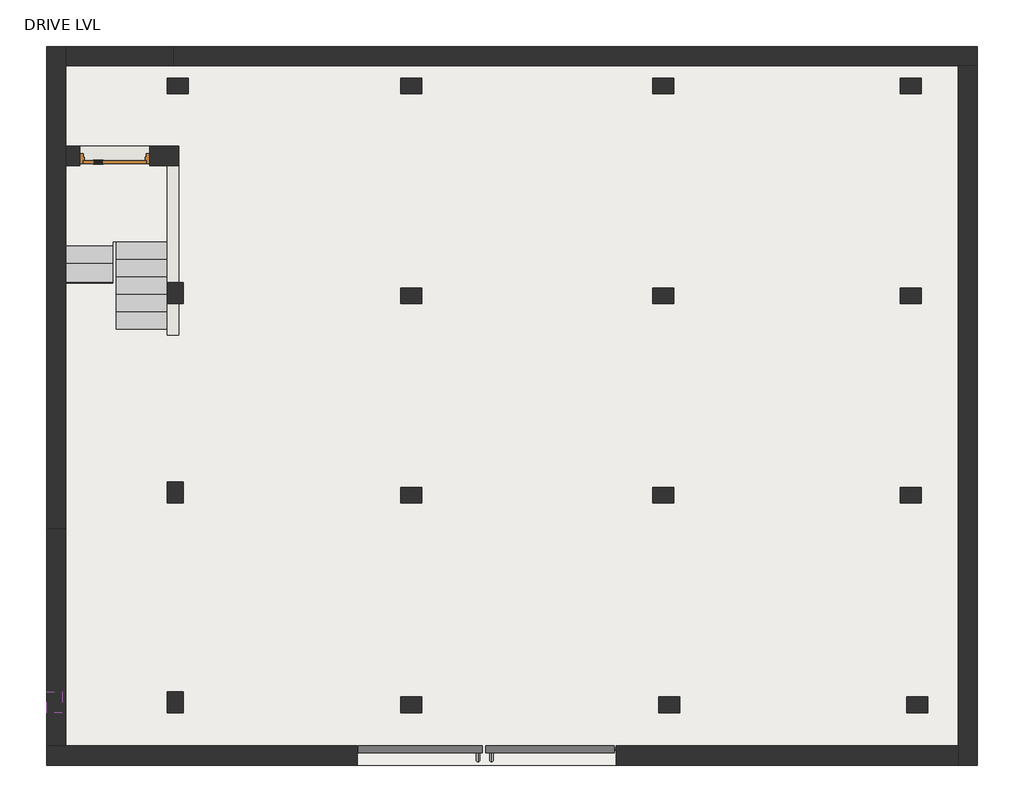
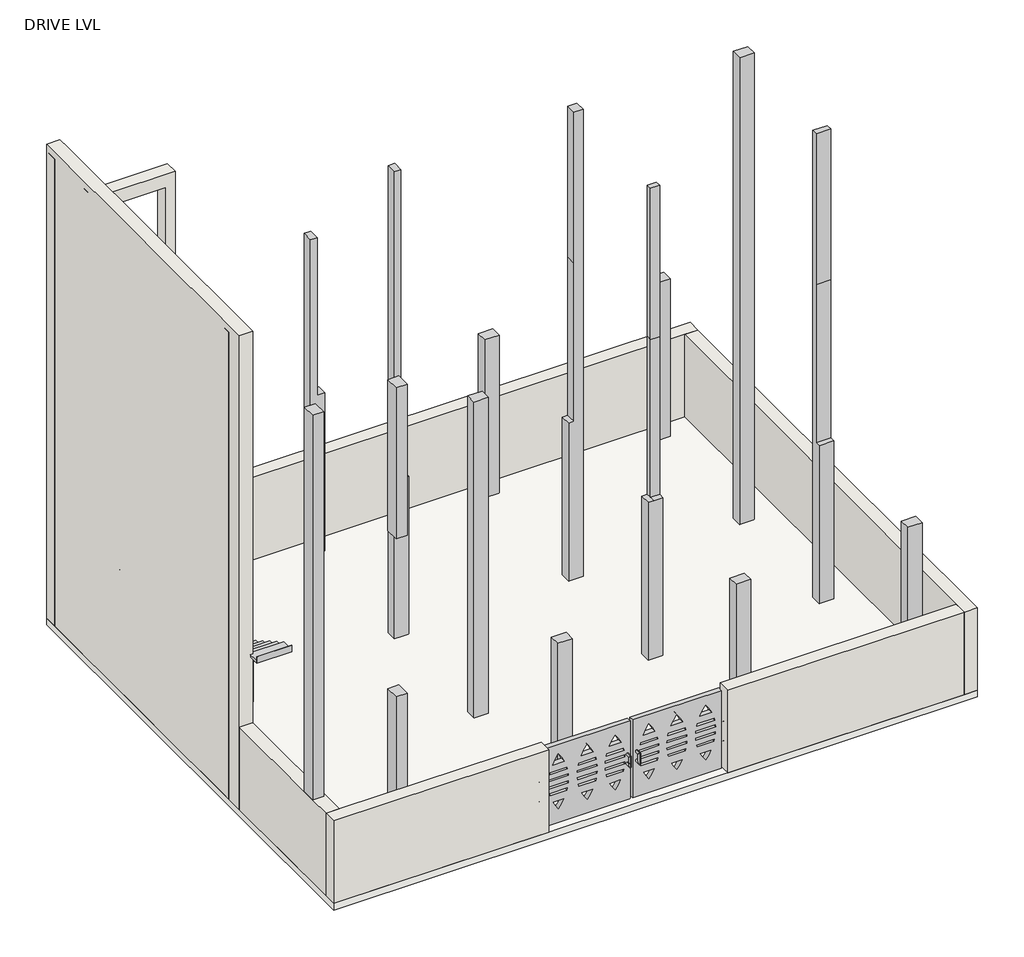
# One storey, incomplete: 21 columns, 8 walls, 2 slabs, 2 stair flights, 1 door, 1 proxy.
"""IFC4 building model written with IfcOpenShell, lengths in millimetres."""

from ifc_helpers import new_model, si_unit, frame, origin, origin_with_axes, place, context, project, spatial, polyline, outline, extrude, faceted_brep, transform, mapped, element, save
from components import generic_models_afecbd1f, column_4e4144c7, door_52fb15b9, non_monolithic_landing_83642a75, stair_flight_3ae1c9df, stair_flight_47155580

model = new_model("IFC4")

# Units and contexts
model_context = context("Model", 3, world=origin())
ifc_project = project(units=[si_unit("LENGTHUNIT", "METRE", prefix="MILLI")], contexts=[model_context])

# Site, building, storey
site = spatial("IfcSite", under=ifc_project)
building = spatial("IfcBuilding", under=site)
storey = spatial("IfcBuildingStorey", under=building, Name="DRIVE LVL", Elevation=0.0)

# Proxy
placement = place(None, origin())
generic_models_shape = generic_models_afecbd1f(model_context)
element("IfcBuildingElementProxy", 1, Name="Generic Models", at=placement, inside=storey, context=model_context, shape_type="MappedRepresentation", body=[
    mapped(generic_models_shape, transform((-1025.2155596, -1244.2923147, 0.0), x_axis=(1.0, 0.0, 0.0), y_axis=(0.0, 1.0, 0.0), z_axis=(0.0, 0.0, 1.0))),
])

# Columns
element("IfcColumn", 2, ObjectType="Rectangular Column : 24\" x 24\" 2", at=placement, inside=storey, context=model_context, shape_type="SweptSolid", body=[
    extrude(outline(polyline([(5711.1209761, -533.0923147), (5711.1209761, -761.6923147), (5406.3209761, -761.6923147), (5406.3209761, -533.0923147), (5711.1209761, -533.0923147)])), origin_with_axes(), (0.0, 0.0, 1.0), 3505.2),
])
element("IfcColumn", 3, ObjectType="Rectangular Column : 24\" x 24\" 2", at=placement, inside=storey, context=model_context, shape_type="SweptSolid", body=[
    extrude(outline(polyline([(2110.3088354, -533.0923147), (2110.3088354, -761.6923147), (1805.5088354, -761.6923147), (1805.5088354, -533.0923147), (2110.3088354, -533.0923147)])), origin_with_axes(), (0.0, 0.0, 1.0), 3505.2),
])
element("IfcColumn", 4, ObjectType="Rectangular Column : 24\" x 24\" 2", at=placement, inside=storey, context=model_context, shape_type="SweptSolid", body=[
    extrude(outline(polyline([(-1634.8155596, -533.0923147), (-1634.8155596, -761.6923147), (-1939.6155596, -761.6923147), (-1939.6155596, -533.0923147), (-1634.8155596, -533.0923147)])), origin_with_axes(), (0.0, 0.0, 1.0), 3505.2),
])
element("IfcColumn", 5, ObjectType="Rectangular Column : 24\" x 24\" 2", at=placement, inside=storey, context=model_context, shape_type="SweptSolid", body=[
    extrude(outline(polyline([(-1634.8155596, 2514.9076853), (-1634.8155596, 2286.3076853), (-1939.6155596, 2286.3076853), (-1939.6155596, 2514.9076853), (-1634.8155596, 2514.9076853)])), origin_with_axes(), (0.0, 0.0, 1.0), 7010.4),
])
element("IfcColumn", 6, ObjectType="Rectangular Column : 24\" x 24\" 2", at=placement, inside=storey, context=model_context, shape_type="SweptSolid", body=[
    extrude(outline(polyline([(0.0, -1939.6155596), (0.0, -1634.8155596), (3505.2, -1634.8155596), (3505.2, -1799.9155596), (7010.4, -1799.9155596), (10363.2, -1799.9155596), (10363.2, -1939.6155596), (0.0, -1939.6155596)])), frame((0.0, 5181.9076853, 0.0), z_axis=(0.0, 1.0, 0.0), x_axis=(0.0, 0.0, 1.0)), (0.0, 0.0, 1.0), 228.6),
])
element("IfcColumn", 7, ObjectType="Rectangular Column : 24\" x 24\" 2", at=placement, inside=storey, context=model_context, shape_type="SweptSolid", body=[
    extrude(outline(polyline([(0.0, 1717.9844404), (0.0, 2022.7844404), (10363.2, 2022.7844404), (10363.2, 1832.2844404), (7010.4, 1832.2844404), (3505.2, 1832.2844404), (3505.2, 1717.9844404), (0.0, 1717.9844404)])), frame((0.0, 5181.9076853, 0.0), z_axis=(0.0, 1.0, 0.0), x_axis=(0.0, 0.0, 1.0)), (0.0, 0.0, 1.0), 228.6),
])
element("IfcColumn", 8, ObjectType="Rectangular Column : 24\" x 24\" 2", at=placement, inside=storey, context=model_context, shape_type="SweptSolid", body=[
    extrude(outline(polyline([(2022.7844404, 8458.5076853), (2022.7844404, 8229.9076853), (1717.9844404, 8229.9076853), (1717.9844404, 8458.5076853), (2022.7844404, 8458.5076853)])), origin_with_axes(), (0.0, 0.0, 1.0), 3505.2),
])
element("IfcColumn", 9, ObjectType="Rectangular Column : 24\" x 24\" 2", at=placement, inside=storey, context=model_context, shape_type="SweptSolid", body=[
    extrude(outline(polyline([(0.0, -1939.6155596), (0.0, -1634.8155596), (3505.2, -1634.8155596), (3505.2, -1799.9155596), (7010.4, -1799.9155596), (7010.4, -1939.6155596), (0.0, -1939.6155596)])), frame((0.0, 8229.9076853, 0.0), z_axis=(0.0, 1.0, 0.0), x_axis=(0.0, 0.0, 1.0)), (0.0, 0.0, 1.0), 228.6),
])
element("IfcColumn", 10, ObjectType="Rectangular Column : 24\" x 24\" 2", at=placement, inside=storey, context=model_context, shape_type="SweptSolid", body=[
    extrude(outline(polyline([(0.0, -5330.5155596), (0.0, -5025.7155596), (7010.4, -5025.7155596), (7010.4, -5101.9155596), (3505.2, -5101.9155596), (3505.2, -5330.5155596), (0.0, -5330.5155596)])), frame((0.0, 8229.9076853, 0.0), z_axis=(0.0, 1.0, 0.0), x_axis=(0.0, 0.0, 1.0)), (0.0, 0.0, 1.0), 228.6),
])
element("IfcColumn", 11, ObjectType="Rectangular Column : 24\" x 24\" 2", at=placement, inside=storey, context=model_context, shape_type="SweptSolid", body=[
    extrude(outline(polyline([(-7083.1155596, 8915.7076853), (-6854.5155596, 8915.7076853), (-6854.5155596, 8610.9076853), (-7083.1155596, 8610.9076853), (-7083.1155596, 8915.7076853)])), origin_with_axes(), (0.0, 0.0, 1.0), 10363.2),
])
element("IfcColumn", 12, ObjectType="Rectangular Column : 24\" x 24\" 2", at=placement, inside=storey, context=model_context, shape_type="SweptSolid", body=[
    extrude(outline(polyline([(-7083.1155596, 7544.1076853), (-6854.5155596, 7544.1076853), (-6854.5155596, 7239.3076853), (-7083.1155596, 7239.3076853), (-7083.1155596, 7544.1076853)])), origin_with_axes(), (0.0, 0.0, 1.0), 10363.2),
])
element("IfcColumn", 13, ObjectType="Rectangular Column : 24\" x 24\" 2", at=placement, inside=storey, context=model_context, shape_type="SweptSolid", body=[
    extrude(outline(polyline([(0.0, -5101.9155596), (3505.2, -5101.9155596), (3505.2, -5330.5155596), (1066.8, -5330.5155596), (1066.8, -5165.4155596), (0.0, -5165.4155596), (0.0, -5101.9155596)])), frame((0.0, 5181.9076853, 0.0), z_axis=(0.0, 1.0, 0.0), x_axis=(0.0, 0.0, 1.0)), (0.0, 0.0, 1.0), 304.8),
])
element("IfcColumn", 14, ObjectType="Rectangular Column : 24\" x 24\" 2", at=placement, inside=storey, context=model_context, shape_type="SweptSolid", body=[
    extrude(outline(polyline([(-5330.5155596, 2591.1076853), (-5101.9155596, 2591.1076853), (-5101.9155596, 2286.3076853), (-5330.5155596, 2286.3076853), (-5330.5155596, 2591.1076853)])), origin_with_axes(), (0.0, 0.0, 1.0), 7010.4),
])
element("IfcColumn", 15, ObjectType="Rectangular Column : 24\" x 24\" 2", at=placement, inside=storey, context=model_context, shape_type="SweptSolid", body=[
    extrude(outline(polyline([(-7083.1155596, 2591.1076853), (-6854.5155596, 2591.1076853), (-6854.5155596, 2286.3076853), (-7083.1155596, 2286.3076853), (-7083.1155596, 2591.1076853)])), origin_with_axes(), (0.0, 0.0, 1.0), 10363.2),
])
element("IfcColumn", 16, ObjectType="Rectangular Column : 24\" x 24\" 2", at=placement, inside=storey, context=model_context, shape_type="Brep", body=[
    faceted_brep([(-7083.1155596, -456.8923147, 10363.2), (-6854.5155596, -456.8923147, 10363.2), (-6854.5155596, -456.8923147, 1828.8), (-7083.1155596, -456.8923147, 1828.8), (-7083.1155596, -456.8923147, 3505.2), (-7083.1155596, -456.8923147, 3810.0), (-7083.1155596, -456.8923147, 7010.4), (-7083.1155596, -456.8923147, 7315.2), (-6854.5155596, -761.6923147, 10363.2), (-6854.5155596, -761.6923147, 1828.8), (-7083.1155596, -761.6923147, 10363.2), (-7083.1155596, -761.6923147, 8077.2), (-7083.1155596, -761.6923147, 7010.4), (-7083.1155596, -761.6923147, 4572.0), (-7083.1155596, -761.6923147, 3505.2), (-7083.1155596, -761.6923147, 1828.8)], [[[0, 1, 2, 3, 4, 5, 6, 7]], [[1, 8, 9, 2]], [[8, 10, 11, 12, 13, 14, 15, 9]], [[10, 0, 7, 6, 5, 4, 3, 15, 14, 13, 12, 11]], [[1, 0, 10, 8]], [[3, 2, 9, 15]]]),
])
element("IfcColumn", 17, ObjectType="Rectangular Column : 24\" x 24\" 2", at=placement, inside=storey, context=model_context, shape_type="SweptSolid", body=[
    extrude(outline(polyline([(-5330.5155596, -456.8923147), (-5101.9155596, -456.8923147), (-5101.9155596, -761.6923147), (-5330.5155596, -761.6923147), (-5330.5155596, -456.8923147)])), origin_with_axes(), (0.0, 0.0, 1.0), 3505.2),
    extrude(outline(polyline([(-5330.5155596, -456.8923147), (-5101.9155596, -456.8923147), (-5101.9155596, -761.6923147), (-5330.5155596, -761.6923147), (-5330.5155596, -456.8923147)])), frame((0.0, 0.0, 7010.4), z_axis=(0.0, 0.0, 1.0), x_axis=(1.0, 0.0, 0.0)), (0.0, 0.0, 1.0), 3352.8),
])
element("IfcColumn", 18, ObjectType="Rectangular Column : 24\" x 24\" 2", at=placement, inside=storey, context=model_context, shape_type="SweptSolid", body=[
    extrude(outline(polyline([(2514.9076853, 0.0), (2286.3076853, 0.0), (2286.3076853, 3505.2), (2400.6076853, 3505.2), (2400.6076853, 7010.4), (2400.6076853, 10363.2), (2514.9076853, 10363.2), (2514.9076853, 0.0)])), frame((5307.0165832, 0.0, 0.0), z_axis=(1.0, 0.0, 0.0), x_axis=(0.0, 1.0, 0.0)), (0.0, 0.0, 1.0), 304.8),
])
element("IfcColumn", 19, ObjectType="Rectangular Column : 24\" x 24\" 2", at=placement, inside=storey, context=model_context, shape_type="SweptSolid", body=[
    extrude(outline(polyline([(5307.0165832, 8229.9076853), (5307.0165832, 8458.5076853), (5611.8165832, 8458.5076853), (5611.8165832, 8229.9076853), (5307.0165832, 8229.9076853)])), origin_with_axes(), (0.0, 0.0, 1.0), 3505.2),
])
element("IfcColumn", 20, ObjectType="Rectangular Column : 24\" x 24\" 2", at=placement, inside=storey, context=model_context, shape_type="Brep", body=[
    faceted_brep([(2022.7844404, 2514.9076853, 0.0), (2022.7844404, 2286.3076853, 0.0), (1717.9844404, 2286.3076853, 0.0), (1717.9844404, 2514.9076853, 0.0), (2022.7844404, 2514.9076853, 10363.2), (2022.7844404, 2400.6076853, 10363.2), (2022.7844404, 2400.6076853, 7010.4), (2022.7844404, 2400.6076853, 3505.2), (2022.7844404, 2286.3076853, 3505.2), (1717.9844404, 2514.9076853, 3505.2), (1832.2844404, 2514.9076853, 3505.2), (1832.2844404, 2514.9076853, 7010.4), (1832.2844404, 2514.9076853, 10363.2), (1832.2844404, 2400.6076853, 10363.2), (1832.2844404, 2400.6076853, 3505.2), (1832.2844404, 2400.6076853, 7010.4), (1717.9844404, 2286.3076853, 3505.2), (1832.2844404, 2286.3076853, 3505.2)], [[[0, 1, 2, 3]], [[1, 0, 4, 5, 6, 7, 8]], [[0, 3, 9, 10, 11, 12, 4]], [[4, 12, 13, 5]], [[11, 10, 14, 15]], [[16, 17, 14, 10, 9]], [[14, 7, 6, 15]], [[7, 14, 17, 8]], [[3, 2, 16, 9]], [[2, 1, 8, 17, 16]], [[12, 11, 15, 13]], [[6, 5, 13, 15]]]),
])
element("IfcColumn", 21, ObjectType="Rectangular Column : 24\" x 24\" 2", at=placement, inside=storey, context=model_context, shape_type="SweptSolid", body=[
    extrude(outline(polyline([(-1939.6155596, -761.6923147), (-1939.6155596, -533.0923147), (-1634.8155596, -533.0923147), (-1634.8155596, -761.6923147), (-1939.6155596, -761.6923147)])), origin_with_axes(), (0.0, 0.0, 1.0), 3505.2),
])
column_shape = column_4e4144c7(model_context)
element("IfcColumn", 22, ObjectType="Rectangular Column : 24\" x 24\" 2", at=placement, inside=storey, context=model_context, shape_type="MappedRepresentation", body=[
    mapped(column_shape, transform((5459.4165832, 5296.2076853, 0.0), x_axis=(-1.0, 0.0, 0.0), y_axis=(0.0, -1.0, 0.0), z_axis=(0.0, 0.0, 1.0))),
])

# Door
door_shape = door_52fb15b9(model_context)
element("IfcDoor", 23, ObjectType="Door-Passage-Single-Vision_Two_Lite : 36\" x 84\"", at=placement, inside=storey, context=model_context, shape_type="MappedRepresentation", body=[
    mapped(door_shape, transform((-6092.5155596, 7334.5576853, 825.5), x_axis=(1.0, 0.0, 0.0), y_axis=(0.0, 1.0, 0.0), z_axis=(0.0, 0.0, 1.0))),
])

# Slabs
element("IfcSlab", 24, ObjectType="Generic - 6\"", at=placement, inside=storey, context=model_context, shape_type="SweptSolid", body=[
    extrude(outline(polyline([(6429.6844404, 8915.7076853), (6429.6844404, -1523.6923147), (-7083.1155596, -1523.6923147), (-7083.1155596, 8915.7076853), (6429.6844404, 8915.7076853)])), frame((0.0, 0.0, -152.4), z_axis=(0.0, 0.0, 1.0), x_axis=(1.0, 0.0, 0.0)), (0.0, 0.0, 1.0), 152.4),
])
non_monolithic_landing_shape = non_monolithic_landing_83642a75(model_context)
element("IfcSlab", 25, ObjectType="Non-Monolithic Landing", at=placement, inside=storey, context=model_context, shape_type="MappedRepresentation", body=[
    mapped(non_monolithic_landing_shape, transform((0.0, 0.0, 0.0), x_axis=(1.0, 0.0, 0.0), y_axis=(0.0, 1.0, 0.0), z_axis=(0.0, 0.0, 1.0))),
])

# Stair flights
stair_flight_shape = stair_flight_3ae1c9df(model_context)
element("IfcStairFlight", 26, ObjectType="2\" Tread 1\" Nosing 1/4\" Riser", at=placement, inside=storey, context=model_context, shape_type="MappedRepresentation", body=[
    mapped(stair_flight_shape, transform((0.0, 0.0, 0.0), x_axis=(1.0, 0.0, 0.0), y_axis=(0.0, 1.0, 0.0), z_axis=(0.0, 0.0, 1.0))),
])
stair_flight_2_shape = stair_flight_47155580(model_context)
element("IfcStairFlight", 27, ObjectType="2\" Tread 1\" Nosing 1/4\" Riser", at=placement, inside=storey, context=model_context, shape_type="MappedRepresentation", body=[
    mapped(stair_flight_2_shape, transform((0.0, 0.0, 0.0), x_axis=(1.0, 0.0, 0.0), y_axis=(0.0, 1.0, 0.0), z_axis=(0.0, 0.0, 1.0))),
])

# Walls
element("IfcWall", 28, ObjectType="4", at=placement, inside=storey, context=model_context, shape_type="Brep", body=[
    faceted_brep([(-5330.5155596, 7188.5076853, 0.0), (-5330.5155596, 4727.0578046, 0.0), (-5330.5155596, 4727.0578046, 1066.8), (-5330.5155596, 5181.9076853, 1066.8), (-5330.5155596, 5486.7076853, 1066.8), (-5330.5155596, 7188.5076853, 1066.8), (-5165.4155596, 7188.5076853, 0.0), (-5165.4155596, 7188.5076853, 1066.8), (-5165.4155596, 5486.7076853, 1066.8), (-5165.4155596, 5181.9076853, 1066.8), (-5165.4155596, 4727.0578046, 1066.8), (-5165.4155596, 4727.0578046, 0.0), (-5165.4155596, 5181.9076853, 0.0), (-5165.4155596, 5486.7076853, 0.0)], [[[0, 1, 2, 3, 4, 5]], [[6, 7, 8, 9, 10, 11, 12, 13]], [[1, 0, 6, 13, 12, 11]], [[2, 1, 11, 10]], [[5, 4, 3, 2, 10, 9, 8, 7]], [[0, 5, 7, 6]]]),
])
element("IfcWall", 29, ObjectType="9", at=placement, inside=storey, context=model_context, shape_type="Brep", body=[
    faceted_brep([(-6803.7155596, 8636.3076853, 0.0), (-5241.6155596, 8636.3076853, 0.0), (-5241.6155596, 8636.3076853, 1828.8), (-5241.6155596, 8636.3076853, 3505.2), (-5101.9155596, 8636.3076853, 3505.2), (-5101.9155596, 8636.3076853, 7010.4), (-5381.3155596, 8636.3076853, 7010.4), (-6803.7155596, 8636.3076853, 7010.4), (-6803.7155596, 8915.7076853, 0.0), (-6803.7155596, 8915.7076853, 7010.4), (-5101.9155596, 8915.7076853, 7010.4), (-5101.9155596, 8915.7076853, 3505.2), (-5241.6155596, 8915.7076853, 3505.2), (-5241.6155596, 8915.7076853, 1828.8), (-5241.6155596, 8915.7076853, 0.0), (-5101.9155596, 8750.6076853, 7010.4), (-5101.9155596, 8750.6076853, 3505.2)], [[[0, 1, 2, 3, 4, 5, 6, 7]], [[8, 9, 10, 11, 12, 13, 14]], [[1, 0, 8, 14]], [[7, 6, 5, 15, 10, 9]], [[0, 7, 9, 8]], [[3, 2, 1, 14, 13, 12]], [[11, 16, 4, 3, 12]], [[5, 4, 16, 11, 10, 15]]]),
])
element("IfcWall", 30, ObjectType="9", at=placement, inside=storey, context=model_context, shape_type="Brep", body=[
    faceted_brep([(-6803.7155596, 7188.5076853, 0.0), (-5330.5155596, 7188.5076853, 0.0), (-5165.4155596, 7188.5076853, 0.0), (-5165.4155596, 7188.5076853, 1066.8), (-5165.4155596, 7188.5076853, 3505.2), (-5381.3155596, 7188.5076853, 3505.2), (-5381.3155596, 7188.5076853, 10364.7228861), (-6803.7155596, 7188.5076853, 10364.7228861), (-5584.5155596, 7188.5076853, 6565.9), (-5584.5155596, 7188.5076853, 4330.7), (-6600.5155596, 7188.5076853, 4330.7), (-6600.5155596, 7188.5076853, 6565.9), (-5584.5155596, 7188.5076853, 3060.7), (-5584.5155596, 7188.5076853, 825.5), (-6600.5155596, 7188.5076853, 825.5), (-6600.5155596, 7188.5076853, 3060.7), (-5584.5155596, 7188.5076853, 10071.1), (-5584.5155596, 7188.5076853, 7835.9), (-6600.5155596, 7188.5076853, 7835.9), (-6600.5155596, 7188.5076853, 10071.1), (-5165.4155596, 7467.9076853, 0.0), (-6803.7155596, 7467.9076853, 0.0), (-6803.7155596, 7467.9076853, 10364.7228861), (-5381.3155596, 7467.9076853, 10364.7228861), (-5381.3155596, 7467.9076853, 3505.2), (-5165.4155596, 7467.9076853, 3505.2), (-5584.5155596, 7467.9076853, 4330.7), (-5584.5155596, 7467.9076853, 6565.9), (-6600.5155596, 7467.9076853, 6565.9), (-6600.5155596, 7467.9076853, 4330.7), (-5584.5155596, 7467.9076853, 825.5), (-5584.5155596, 7467.9076853, 3060.7), (-6600.5155596, 7467.9076853, 3060.7), (-6600.5155596, 7467.9076853, 825.5), (-5584.5155596, 7467.9076853, 7835.9), (-5584.5155596, 7467.9076853, 10071.1), (-6600.5155596, 7467.9076853, 10071.1), (-6600.5155596, 7467.9076853, 7835.9)], [[[0, 1, 2, 3, 4, 5, 6, 7], [8, 9, 10, 11], [12, 13, 14, 15], [16, 17, 18, 19]], [[20, 21, 22, 23, 24, 25], [26, 27, 28, 29], [30, 31, 32, 33], [34, 35, 36, 37]], [[2, 1, 0, 21, 20]], [[7, 6, 23, 22]], [[0, 7, 22, 21]], [[26, 9, 8, 27]], [[27, 8, 11, 28]], [[28, 11, 10, 29]], [[9, 26, 29, 10]], [[31, 30, 13, 12]], [[32, 31, 12, 15]], [[33, 32, 15, 14]], [[30, 33, 14, 13]], [[35, 34, 17, 16]], [[36, 35, 16, 19]], [[37, 36, 19, 18]], [[34, 37, 18, 17]], [[5, 4, 25, 24]], [[2, 20, 25, 4, 3]], [[23, 6, 5, 24]]]),
])
element("IfcWall", 31, ObjectType="9", at=placement, inside=storey, context=model_context, shape_type="Brep", body=[
    faceted_brep([(-5241.6155596, 8636.3076853, 0.0), (6150.2844404, 8636.3076853, 0.0), (6429.6844404, 8636.3076853, 0.0), (6429.6844404, 8636.3076853, 1828.8), (6150.2844404, 8636.3076853, 1828.8), (-5241.6155596, 8636.3076853, 1828.8), (-5241.6155596, 8915.7076853, 0.0), (-5241.6155596, 8915.7076853, 1828.8), (6429.6844404, 8915.7076853, 1828.8), (6429.6844404, 8915.7076853, 0.0)], [[[0, 1, 2, 3, 4, 5]], [[6, 7, 8, 9]], [[2, 1, 0, 6, 9]], [[5, 4, 3, 8, 7]], [[0, 5, 7, 6]], [[3, 2, 9, 8]]]),
])
element("IfcWall", 32, ObjectType="9", at=placement, inside=storey, context=model_context, shape_type="Brep", body=[
    faceted_brep([(6150.2844404, 8636.3076853, 0.0), (6150.2844404, -1244.2923147, 0.0), (6150.2844404, -1523.6923147, 0.0), (6150.2844404, -1523.6923147, 1828.8), (6150.2844404, -1244.2923147, 1828.8), (6150.2844404, 8636.3076853, 1828.8), (6429.6844404, 8636.3076853, 0.0), (6429.6844404, 8636.3076853, 1828.8), (6429.6844404, -1523.6923147, 1828.8), (6429.6844404, -1523.6923147, 0.0)], [[[0, 1, 2, 3, 4, 5]], [[6, 7, 8, 9]], [[2, 1, 0, 6, 9]], [[5, 4, 3, 8, 7]], [[0, 5, 7, 6]], [[3, 2, 9, 8]]]),
])
element("IfcWall", 33, ObjectType="9", at=placement, inside=storey, context=model_context, shape_type="Brep", body=[
    faceted_brep([(6150.2844404, -1244.2923147, 1828.8), (6150.2844404, -1244.2923147, 0.0), (1189.6442362, -1244.2923147, 0.0), (1189.6442362, -1244.2923147, 1828.8), (6150.2844404, -1523.6923147, 0.0), (6150.2844404, -1523.6923147, 1828.8), (1189.6442362, -1523.6923147, 1828.8), (1189.6442362, -1523.6923147, 0.0)], [[[0, 1, 2, 3]], [[4, 5, 6, 7]], [[1, 4, 7, 2]], [[5, 0, 3, 6]], [[1, 0, 5, 4]], [[3, 2, 7, 6]]]),
    faceted_brep([(-7083.1155596, -1244.2923147, 0.0), (-7083.1155596, -1244.2923147, 1828.8), (-6803.7155596, -1244.2923147, 1828.8), (-2569.5557638, -1244.2923147, 1828.8), (-2569.5557638, -1244.2923147, 0.0), (-6803.7155596, -1244.2923147, 0.0), (-7083.1155596, -1523.6923147, 1828.8), (-7083.1155596, -1523.6923147, 0.0), (-2569.5557638, -1523.6923147, 0.0), (-2569.5557638, -1523.6923147, 1828.8)], [[[0, 1, 2, 3, 4, 5]], [[6, 7, 8, 9]], [[7, 0, 5, 4, 8]], [[1, 6, 9, 3, 2]], [[1, 0, 7, 6]], [[4, 3, 9, 8]]]),
])
element("IfcWall", 34, ObjectType="9", at=placement, inside=storey, context=model_context, shape_type="Brep", body=[
    faceted_brep([(-6803.7155596, -1244.2923147, 0.0), (-6803.7155596, 1905.3076853, 0.0), (-6803.7155596, 1905.3076853, 1828.8), (-6803.7155596, -1244.2923147, 1828.8), (-7083.1155596, -1244.2923147, 0.0), (-7083.1155596, -1244.2923147, 1828.8), (-7083.1155596, -761.6923147, 1828.8), (-7083.1155596, -456.8923147, 1828.8), (-7083.1155596, 1905.3076853, 1828.8), (-7083.1155596, 1905.3076853, 0.0)], [[[0, 1, 2, 3]], [[4, 5, 6, 7, 8, 9]], [[1, 0, 4, 9]], [[2, 1, 9, 8]], [[3, 2, 8, 7, 6, 5]], [[0, 3, 5, 4]]]),
])
element("IfcWall", 35, ObjectType="9 2", at=placement, inside=storey, context=model_context, shape_type="Brep", body=[
    faceted_brep([(-7083.1155596, 8915.7076853, 10515.6), (-7083.1155596, 8915.7076853, 0.0), (-7083.1155596, 1905.3076853, 0.0), (-7083.1155596, 1905.3076853, 1828.8), (-7083.1155596, 1905.3076853, 3505.2), (-7083.1155596, 1905.3076853, 3810.0), (-7083.1155596, 1905.3076853, 7010.4), (-7083.1155596, 1905.3076853, 7315.2), (-7083.1155596, 1905.3076853, 10515.6), (-6803.7155596, 8915.7076853, 0.0), (-6803.7155596, 8915.7076853, 7010.4), (-6803.7155596, 8915.7076853, 10515.6), (-6803.7155596, 8636.3076853, 10515.6), (-6803.7155596, 1905.3076853, 10515.6), (-6803.7155596, 1905.3076853, 1828.8), (-6803.7155596, 1905.3076853, 0.0), (-6803.7155596, 7188.5076853, 0.0), (-6803.7155596, 7467.9076853, 0.0), (-6803.7155596, 8636.3076853, 0.0)], [[[0, 1, 2, 3, 4, 5, 6, 7, 8]], [[9, 10, 11, 12, 13, 14, 15, 16, 17, 18]], [[2, 1, 9, 18, 17, 16, 15]], [[0, 8, 13, 12, 11]], [[0, 11, 10, 9, 1]], [[2, 15, 14, 13, 8, 7, 6, 5, 4, 3]]]),
])

save(model, "model.ifc")

# Revit data of these elements
# Type
#   Default Elevation = 0
# Type "Rectangular Column : 24\" x 24\" 2"
#   Assembly Code = "B1010200"
#   Depth = 0' - 9"
#   Offset Base = 0' - 0"
#   Offset Top = 0' - 0"
#   Width = 1' - 0"
#   Material = none
# Type "Door-Passage-Single-Vision_Two_Lite : 36\" x 84\""
#   Type Mark = "9"
#   Assembly Code = "B2030100"
#   Analytic Construction = "Wooden"
#   Thickness = 0' - 1 3/4"
#   Thermal Resistance (R) = 2.5876 (h·ft²·°F)/BTU
#   Swing Angle [instance default] = 90.00°
#   Strike Height = 3' - 4"
#   Rough Width [instance default] = 3' - 4"
#   Rough Height [instance default] = 7' - 4"
#   MF Opening Height [instance default] = 0' - 4"
#   MF Opening Width [instance default] = 0' - 4"
#   Heat Transfer Coefficient (U) = 0.3865 BTU/(h·ft²·°F)
#   Inset Calculate [instance default] = 0' - 4"
#   Masonry Inset [instance default] = 0' - 1"
#   Height = 7' - 0"
#   Width = 3' - 0"
#   Masonry Frame Depth = 0' - 5 3/4"
#   Masonry Frame [instance default] = yes
#   Function = 1
#   Dry Wall Frame [instance default] = no
#   Panel Material = Wood - Birch
#   Glazing = Glass
#   Glass Stop Material = Metal - Paint Finish - Grey
#   Frame Material = Metal - Paint Finish - Grey
#   Door Handle Material = Aluminum
#   Visual Light Transmittance = 0
#   Solar Heat Gain Coefficient = 0
#   Wall Closure = (empty or 0)
# Type "Generic - 6\""
#   Assembly Code = "B1010"
#   Function = 0
#   Layers, outside or top first: 0' - 6" no material (function 1)
# Type "4"
#   Assembly Code = "B2010"
#   Layers, outside or top first: 0' - 1" "Gypsum Wall Board" (function 1); 0' - 4 1/2" no material (function 1); 0' - 1" "Gypsum Wall Board" (function 1)
# Type "9"
#   Assembly Code = "B2010"
#   Layers, outside or top first: 0' - 1" "Gypsum Wall Board" (function 1); 0' - 9" no material (function 1); 0' - 1" "Gypsum Wall Board" (function 1)
# Type "9 2"
#   Assembly Code = "B2010"
#   Layers, outside or top first: 0' - 1" "Gypsum Wall Board" (function 1); 0' - 9" no material (function 1); 0' - 1" "Gypsum Wall Board" (function 1)
# Element 1 (IfcBuildingElementProxy)
#   Phase Created = New Construction
#   Materials on its faces: "GATE"
# Elements 2, 3, 4, 5, 6, 7, 8, 9, 10, 13, 14, 16, 17, 18, 19, 20, 21 (IfcColumn, "Rectangular Column : 24\" x 24\" 2")
#   Phase Created = New Construction
#   Materials on its faces: "Gypsum Wall Board", "Default Wall"
# Elements 11, 12, 15, 22 (IfcColumn, "Rectangular Column : 24\" x 24\" 2")
#   Phase Created = New Construction
# Element 23 (IfcDoor, "Door-Passage-Single-Vision_Two_Lite : 36\" x 84\"")
#   Swing Angle = 90.00°
#   Rough Width = 3' - 4"
#   Rough Height = 7' - 4"
#   Masonry Inset = 0' - 1"
#   MF Opening Width = 0' - 4"
#   MF Opening Height = 0' - 4"
#   Inset Calculate = 0' - 4"
#   Masonry Frame = yes
#   Dry Wall Frame = no
#   Phase Created = New Construction
#   Materials on its faces: "Metal - Paint Finish - Grey", "Aluminum", "Wood - Birch", "Glass"
# Element 24 (IfcSlab, "Generic - 6\"")
#   Height Offset From Level = 0' - 0"
#   Phase Created = New Construction
#   Materials on its faces: "Default Floor"
# Element 25 (IfcSlab, "Non-Monolithic Landing")
#   Phase Created = New Construction
# Elements 26, 27 (IfcStairFlight, "2\" Tread 1\" Nosing 1/4\" Riser")
#   Phase Created = New Construction
# Element 28 (IfcWall, "4")
#   Top Offset = 0' - 0"
#   Base Offset = 0' - 0"
#   Unconnected Height = 3' - 6"
#   wall height = 3' - 6"
#   Phase Created = New Construction
#   Base Constraint = DRIVE LVL
#   Materials on its faces: "Default Wall", "Gypsum Wall Board"
# Element 29 (IfcWall, "9")
#   Top Offset = 0' - 0"
#   Base Offset = 0' - 0"
#   wall height = 23' - 0"
#   Phase Created = New Construction
#   Base Constraint = DRIVE LVL
#   Top Constraint = SECOND FLOOR LVL
#   Materials on its faces: "Default Wall", "Gypsum Wall Board"
# Element 30 (IfcWall, "9")
#   Top Offset = -0' - 5.94004"
#   Base Offset = 0' - 0"
#   wall height = 34' - 0.05996"
#   Phase Created = New Construction
#   Base Constraint = DRIVE LVL
#   Top Constraint = ROOF LVL
#   Materials on its faces: "Default Wall", "Gypsum Wall Board"
# Elements 31, 32 (IfcWall, "9")
#   Top Offset = 0' - 0"
#   Base Offset = 0' - 0"
#   Unconnected Height = 6' - 0"
#   wall height = 6' - 0"
#   Phase Created = New Construction
#   Base Constraint = DRIVE LVL
#   Materials on its faces: "Gypsum Wall Board", "Default Wall"
# Elements 33, 34 (IfcWall, "9")
#   Top Offset = 0' - 0"
#   Base Offset = 0' - 0"
#   Unconnected Height = 6' - 0"
#   wall height = 6' - 0"
#   Phase Created = New Construction
#   Base Constraint = DRIVE LVL
#   Materials on its faces: "Default Wall", "Gypsum Wall Board"
# Element 35 (IfcWall, "9 2")
#   Top Offset = 0' - 0"
#   Base Offset = 0' - 0"
#   wall height = 34' - 6"
#   Phase Created = New Construction
#   Base Constraint = DRIVE LVL
#   Top Constraint = ROOF LVL
#   Materials on its faces: "Gypsum Wall Board", "Default Wall"
# Materials
#   "Wood - Birch": class "Wood", colour RGB 166 116 52, transparency 0, Cost = 0
#   "Glass": class "Glass", colour RGB 0 128 192, transparency 0.75, Description = "Soda Lime Glass", Cost = 0
#   "Metal - Paint Finish - Grey": class "Paint", colour RGB 104 104 104, transparency 0, Cost = 0
#   "Aluminum": class "Metal", colour RGB 247 247 247, transparency 0, Description = "Aluminum 6061", Cost = 0
#   "Gypsum Wall Board": class "Generic", colour RGB 228 228 228, transparency 0, Description = "Gypsum Wall Board", Cost = 0
#   "GATE": class "Generic", colour RGB 120 120 120, transparency 0, Cost = 0
#   "Default Wall": colour RGB 128 128 128, transparency 0, Cost = 0
#   "Default Floor": colour RGB 128 128 128, transparency 0, Cost = 0
